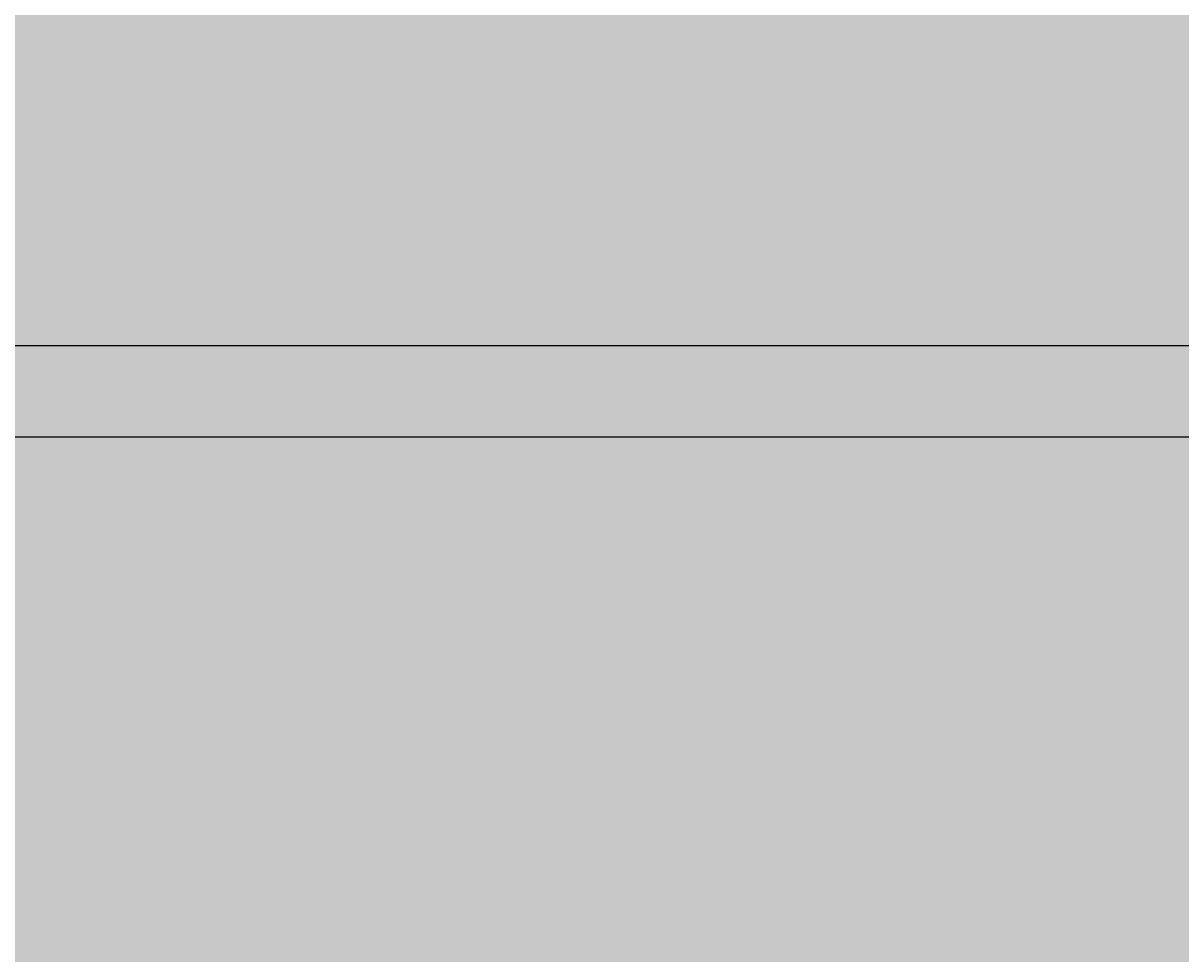
# Model space of a CAD drawing. Units: inches. Extents: x -12 to 334, y -10 to 186.
# Tile 63 of 77: x 184 to 216, y 111 to 137. Entities that reach past the tile are written whole.
import ezdxf

# ---------------------------------------------------------------- set-up
doc = ezdxf.new("R2010")
doc.units = ezdxf.units.IN
doc.header["$MEASUREMENT"] = 0
doc.layers.add('M-DIMS', color=2, linetype='Continuous', lineweight=18)
doc.layers.add('M-EQPM-PATT', color=8, linetype='Continuous', lineweight=18)
doc.styles.get("Standard").update_dxf_attribs({"font": 'arial.ttf'})
doc.dimstyles.get("Standard").update_dxf_attribs({"dimtxt": 0.18, "dimasz": 0.18, "dimexe": 0.18, "dimexo": 0.0625, "dimgap": 0.09, "dimtad": 0, "dimtih": 1, "dimtoh": 1, "dimdec": 4, "dimzin": 0, "dimdsep": 46, "dimtxsty": 'Standard', "dimcen": 0.09, "dimadec": 0, "dimazin": 0, "dimtfac": 1, "dimtdec": 4, "dimtofl": 0, "dimtmove": 0, "dimatfit": 3, "dimfxl": 1, "dimtolj": 1, "dimtzin": 0, "dimarcsym": 0})

# ---------------------------------------------------------------- blocks, each defined once
blk = doc.blocks.new('*D5')
at = {"layer": 'Defpoints', "color": 0, "transparency": 16777216}
for p in [(58.1, 127.708), (58.1, 125.208), (295.976, 125.208)]:
    blk.add_point(p, dxfattribs=at)
at = {"layer": 'M-DIMS', "color": 0, "lineweight": -2, "transparency": 16777216}
for p, q in [((58.163, 127.708), (296.156, 127.708)), ((295.976, 127.528), (295.976, 126.64)), ((295.976, 125.388), (295.976, 126.276)), ((58.163, 125.208), (296.156, 125.208))]:
    blk.add_line(p, q, dxfattribs=at)
at = {"layer": 'M-DIMS', "color": 0, "transparency": 16777216}
for points in [[(295.946, 127.528), (296.006, 127.528), (295.976, 127.708)], [(295.946, 125.388), (296.006, 125.388), (295.976, 125.208)]]:
    blk.add_solid(points, dxfattribs=at)
at = {"layer": 'M-DIMS', "color": 0, "transparency": 16777216, "insert": (295.976, 126.458), "char_height": 0.18, "attachment_point": 5}
blk.add_mtext('\\A1;2.5', dxfattribs=at)
blk = doc.blocks.new('*D40')
at = {"layer": 'Defpoints', "color": 0, "transparency": 16777216}
for p in [(278.229, 116.208), (187.394, 91.899)]:
    blk.add_point(p, dxfattribs=at)
at = {"layer": 'M-DIMS', "color": 0, "lineweight": -2, "transparency": 16777216}
for p, q in [((332.73, 130.793), (278.403, 116.254)), ((187.304, 91.899), (187.484, 91.899)), ((187.394, 91.809), (187.394, 91.989))]:
    blk.add_line(p, q, dxfattribs=at)
at = {"layer": 'M-DIMS', "color": 0, "transparency": 16777216}
blk.add_solid([(278.395, 116.283), (278.411, 116.225), (278.229, 116.208)], dxfattribs=at)
at = {"layer": 'M-DIMS', "color": 0, "transparency": 16777216, "insert": (333.21, 130.793), "char_height": 0.18, "attachment_point": 5}
blk.add_mtext('\\A1;R94.03', dxfattribs=at)

msp = doc.modelspace()

# ---------------------------------------------------------------- hatches: boundary and pattern name
at = {"layer": 'M-EQPM-PATT', "transparency": 33554556}
h = msp.add_hatch(color=256, dxfattribs=at)
h.set_gradient(color1=(248, 206, 179), color2=(248, 206, 179), tint=1)
h.paths.add_polyline_path([(179.7818, 136.8871), (126.9567, 136.8871), (106.1771, 100.8958), (171.5458, 100.8958)])
h.paths.add_polyline_path([(268.3808, 136.9435), (214.0166, 136.9435), (214.0166, 154.8345), (196.3421, 154.8345), (196.3421, 136.8871), (179.7818, 136.8871), (171.5458, 100.8958), (231.7758, 100.8958, -0.4142136), (251.9801, 80.6915), (279.7263, 80.6915, 0.1631825)])

# ---------------------------------------------------------------- dimensions: what is measured, and where the dimension line sits
at = {"layer": 'M-DIMS'}
dim = msp.add_radius_dim(center=(187.3936, 91.8988), mpoint=(278.2291, 116.2078), dimstyle='Standard', override={"dimdec": 2, "dimlfac": 1, "dimrnd": 0, "dimzin": 0, "dimdsep": 46, "dimlunit": 2}, dxfattribs=at)
dim.commit()
dim.dimension.update_dxf_attribs({"geometry": '*D40', "text_midpoint": (332.7304, 130.7932), "dimtype": 164})
dim = msp.add_linear_dim(base=(295.9756, 125.2078), p1=(58.1002, 127.7078), p2=(58.1002, 125.2078), angle=90, dimstyle='Standard', override={"dimdec": 1, "dimlfac": 1, "dimrnd": 0, "dimzin": 0, "dimdsep": 46, "dimlunit": 2}, dxfattribs=at)
dim.commit()
dim.dimension.update_dxf_attribs({"geometry": '*D5', "text_midpoint": (295.9756, 126.4578)})

doc.saveas('drawing.dxf')
